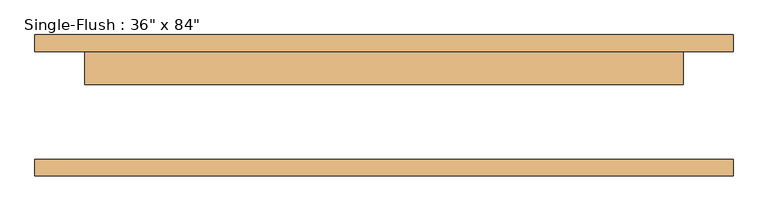
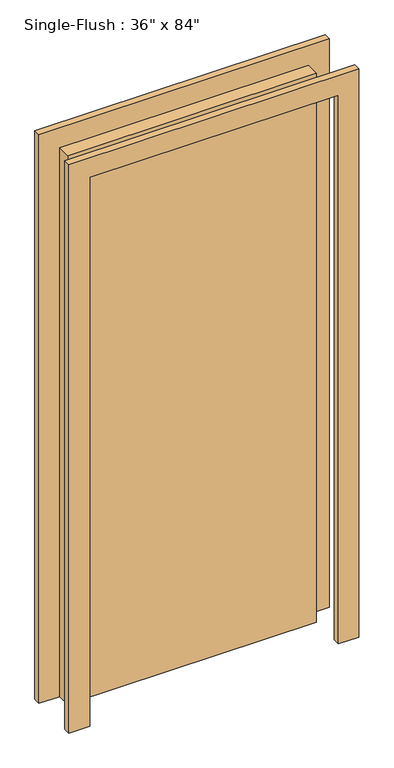
"""IFC4 building model written with IfcOpenShell, lengths in millimetres: door geometry."""

from ifc_helpers import new_model, si_unit, frame, origin, origin_with_axes, place, context, project, spatial, polyline, outline, extrude, source, transform, mapped, element, save


def door_d2d7de5b(model_context):
    return source(origin(), model_context, "Body", "SweptSolid", [
        extrude(outline(polyline([(2209.8, -533.4), (0.0, -533.4), (0.0, -457.2), (2133.6, -457.2), (2133.6, 457.2), (0.0, 457.2), (0.0, 533.4), (2209.8, 533.4), (2209.8, -533.4)])), frame((0.0, 82.55, 0.0), z_axis=(0.0, 1.0, 0.0), x_axis=(0.0, 0.0, 1.0)), (0.0, 0.0, 1.0), 25.4),
        extrude(outline(polyline([(2209.8, 533.4), (2209.8, -533.4), (0.0, -533.4), (0.0, -457.2), (2133.6, -457.2), (2133.6, 457.2), (0.0, 457.2), (0.0, 533.4), (2209.8, 533.4)])), frame((0.0, -107.95, 0.0), z_axis=(0.0, 1.0, 0.0), x_axis=(0.0, 0.0, 1.0)), (0.0, 0.0, 1.0), 25.4),
        extrude(outline(polyline([(457.2, 31.75), (-457.2, 31.75), (-457.2, 82.55), (457.2, 82.55), (457.2, 31.75)])), origin_with_axes(), (0.0, 0.0, 1.0), 2133.6),
    ])


if __name__ == "__main__":
    model = new_model("IFC4")
    model_context = context("Model", 3, world=origin())
    ifc_project = project(units=[si_unit("LENGTHUNIT", "METRE", prefix="MILLI")], contexts=[model_context])
    site = spatial("IfcSite", under=ifc_project)
    building = spatial("IfcBuilding", under=site)
    placement = place(None, origin())
    door_shape = door_d2d7de5b(model_context)
    element("IfcDoor", 1, ObjectType="Single-Flush : 36\" x 84\"", at=placement, inside=building, context=model_context, shape_type="MappedRepresentation", body=[
        mapped(door_shape, transform((0.0, 0.0, 0.0), x_axis=(1.0, 0.0, 0.0), y_axis=(0.0, 1.0, 0.0), z_axis=(0.0, 0.0, 1.0))),
    ])
    save(model, "model.ifc")

# Revit data of these elements
# Type "Single-Flush : 36\" x 84\""
#   Type Mark = "1"
#   Construction Type Id = "MDOOR"
#   Assembly Code = "C1020"
#   Analytic Construction = "Metal"
#   Thickness = 0' - 2"
#   Heat Transfer Coefficient (U) = 0.651978 BTU/(h·ft²·°F)
#   Height = 7' - 0"
#   Trim Projection Ext = 0' - 1"
#   Trim Projection Int = 0' - 1"
#   Trim Width = 0' - 3"
#   Width = 3' - 0"
#   Define Thermal Properties by = 1
#   Define Thermal Properties by = 1
#   Door Material = Door - Panel
#   Frame Material = Door - Frame
#   Visual Light Transmittance = 0
#   Solar Heat Gain Coefficient = 0
#   Function = (empty or 0)
#   Wall Closure = (empty or 0)
# Element 1 (IfcDoor, "Single-Flush : 36\" x 84\"")
#   Materials on its faces: "Door - Frame", "Door - Panel"
# Materials
#   "Door - Panel": class "Wood", colour RGB 210 159 95, transparency 0, Cost = 0
#   "Door - Frame": colour RGB 118 70 51, transparency 0, Cost = 0
